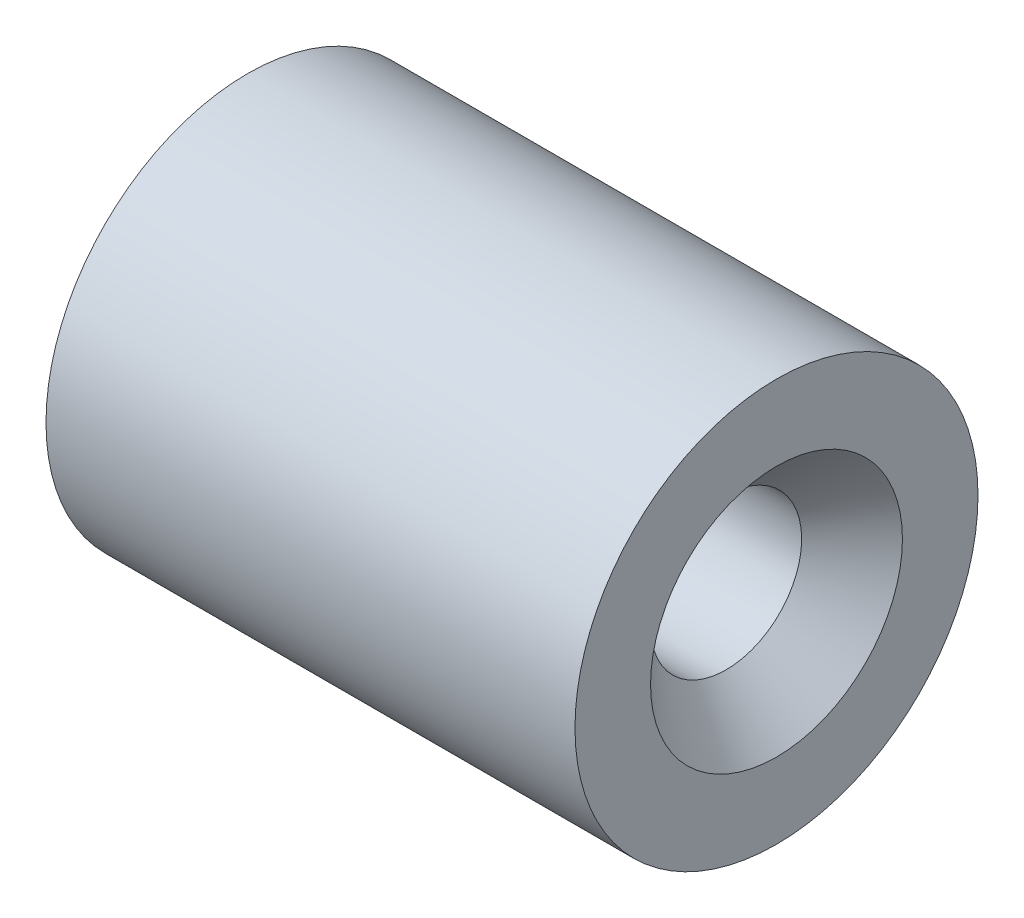
ISO-10303-21;
HEADER;
FILE_DESCRIPTION(('STEP AP214'),'2;1');
FILE_NAME('part.step','',(''),(''),'','','');
FILE_SCHEMA(('AUTOMOTIVE_DESIGN { 1 0 10303 214 1 1 1 1 }'));
ENDSEC;
DATA;
#1=APPLICATION_CONTEXT('core data for automotive mechanical design processes');
#2=APPLICATION_PROTOCOL_DEFINITION('international standard','automotive_design',2000,#1);
#3=PRODUCT_CONTEXT('',#1,'mechanical');
#4=PRODUCT('Part','Part','',(#3));
#5=PRODUCT_RELATED_PRODUCT_CATEGORY('part','',(#4));
#6=PRODUCT_DEFINITION_FORMATION('','',#4);
#7=PRODUCT_DEFINITION_CONTEXT('part definition',#1,'design');
#8=PRODUCT_DEFINITION('design','',#6,#7);
#9=PRODUCT_DEFINITION_SHAPE('','',#8);
#10=(LENGTH_UNIT() NAMED_UNIT(*) SI_UNIT(.MILLI.,.METRE.));
#11=(NAMED_UNIT(*) PLANE_ANGLE_UNIT() SI_UNIT($,.RADIAN.));
#12=(NAMED_UNIT(*) SI_UNIT($,.STERADIAN.) SOLID_ANGLE_UNIT());
#13=UNCERTAINTY_MEASURE_WITH_UNIT(LENGTH_MEASURE(1.E-05),#10,'distance_accuracy_value','');
#14=(GEOMETRIC_REPRESENTATION_CONTEXT(3) GLOBAL_UNCERTAINTY_ASSIGNED_CONTEXT((#13)) GLOBAL_UNIT_ASSIGNED_CONTEXT((#10,
#11,#12)) REPRESENTATION_CONTEXT('',''));
#15=CARTESIAN_POINT('',(0.,0.,0.));
#16=DIRECTION('',(0.,0.,1.));
#17=DIRECTION('',(1.,0.,0.));
#18=AXIS2_PLACEMENT_3D('',#15,#16,#17);
#19=CARTESIAN_POINT('',(0.,16.,0.));
#20=DIRECTION('',(1.,0.,0.));
#21=DIRECTION('',(0.,0.,-1.));
#22=AXIS2_PLACEMENT_3D('',#19,#20,#21);
#23=PLANE('',#22);
#24=CARTESIAN_POINT('',(0.,0.,0.));
#25=DIRECTION('',(1.,0.,0.));
#26=DIRECTION('',(0.,0.,-1.));
#27=AXIS2_PLACEMENT_3D('',#24,#25,#26);
#28=CIRCLE('',#27,16.);
#29=CARTESIAN_POINT('',(0.,0.,-16.));
#30=VERTEX_POINT('',#29);
#31=EDGE_CURVE('E74',#30,#30,#28,.T.);
#32=ORIENTED_EDGE('',*,*,#31,.T.);
#33=EDGE_LOOP('',(#32));
#34=FACE_BOUND('',#33,.T.);
#35=CARTESIAN_POINT('',(0.,0.,0.));
#36=DIRECTION('',(1.,0.,0.));
#37=DIRECTION('',(0.,0.,-1.));
#38=AXIS2_PLACEMENT_3D('',#35,#36,#37);
#39=CIRCLE('',#38,9.99999999999999);
#40=CARTESIAN_POINT('',(0.,0.,-9.99999999999999));
#41=VERTEX_POINT('',#40);
#42=EDGE_CURVE('E49',#41,#41,#39,.T.);
#43=ORIENTED_EDGE('',*,*,#42,.F.);
#44=EDGE_LOOP('',(#43));
#45=FACE_BOUND('',#44,.T.);
#46=ADVANCED_FACE('F39',(#34,#45),#23,.T.);
#47=CARTESIAN_POINT('',(-3.99999999999993,0.,0.));
#48=DIRECTION('',(1.,0.,0.));
#49=DIRECTION('',(0.,0.,-1.));
#50=AXIS2_PLACEMENT_3D('',#47,#48,#49);
#51=CONICAL_SURFACE('',#50,6.,0.785398163397457);
#52=ORIENTED_EDGE('',*,*,#42,.T.);
#53=EDGE_LOOP('',(#52));
#54=FACE_BOUND('',#53,.T.);
#55=CARTESIAN_POINT('',(-3.99999999999993,0.,0.));
#56=DIRECTION('',(1.,0.,0.));
#57=DIRECTION('',(0.,0.,-1.));
#58=AXIS2_PLACEMENT_3D('',#55,#56,#57);
#59=CIRCLE('',#58,6.);
#60=CARTESIAN_POINT('',(-3.99999999999993,0.,-6.));
#61=VERTEX_POINT('',#60);
#62=EDGE_CURVE('E80',#61,#61,#59,.T.);
#63=ORIENTED_EDGE('',*,*,#62,.F.);
#64=EDGE_LOOP('',(#63));
#65=FACE_BOUND('',#64,.T.);
#66=ADVANCED_FACE('F61',(#54,#65),#51,.F.);
#67=CARTESIAN_POINT('',(0.,0.,0.));
#68=DIRECTION('',(1.,0.,0.));
#69=DIRECTION('',(0.,0.,-1.));
#70=AXIS2_PLACEMENT_3D('',#67,#68,#69);
#71=CYLINDRICAL_SURFACE('',#70,6.);
#72=ORIENTED_EDGE('',*,*,#62,.T.);
#73=EDGE_LOOP('',(#72));
#74=FACE_BOUND('',#73,.T.);
#75=CARTESIAN_POINT('',(-38.,0.,0.));
#76=DIRECTION('',(1.,0.,0.));
#77=DIRECTION('',(0.,0.,-1.));
#78=AXIS2_PLACEMENT_3D('',#75,#76,#77);
#79=CIRCLE('',#78,6.);
#80=CARTESIAN_POINT('',(-38.,0.,-6.));
#81=VERTEX_POINT('',#80);
#82=EDGE_CURVE('E76',#81,#81,#79,.T.);
#83=ORIENTED_EDGE('',*,*,#82,.F.);
#84=EDGE_LOOP('',(#83));
#85=FACE_BOUND('',#84,.T.);
#86=ADVANCED_FACE('F69',(#74,#85),#71,.F.);
#87=CARTESIAN_POINT('',(-42.,0.,0.));
#88=DIRECTION('',(-1.,0.,0.));
#89=DIRECTION('',(0.,0.,1.));
#90=AXIS2_PLACEMENT_3D('',#87,#88,#89);
#91=CONICAL_SURFACE('',#90,9.99999999999999,0.78539816339745);
#92=ORIENTED_EDGE('',*,*,#82,.T.);
#93=EDGE_LOOP('',(#92));
#94=FACE_BOUND('',#93,.T.);
#95=CARTESIAN_POINT('',(-42.,0.,0.));
#96=DIRECTION('',(1.,0.,0.));
#97=DIRECTION('',(0.,0.,-1.));
#98=AXIS2_PLACEMENT_3D('',#95,#96,#97);
#99=CIRCLE('',#98,9.99999999999999);
#100=CARTESIAN_POINT('',(-42.,0.,-9.99999999999999));
#101=VERTEX_POINT('',#100);
#102=EDGE_CURVE('E84',#101,#101,#99,.T.);
#103=ORIENTED_EDGE('',*,*,#102,.F.);
#104=EDGE_LOOP('',(#103));
#105=FACE_BOUND('',#104,.T.);
#106=ADVANCED_FACE('F92',(#94,#105),#91,.F.);
#107=CARTESIAN_POINT('',(-42.,9.99999999999999,0.));
#108=DIRECTION('',(-1.,0.,0.));
#109=DIRECTION('',(0.,0.,1.));
#110=AXIS2_PLACEMENT_3D('',#107,#108,#109);
#111=PLANE('',#110);
#112=ORIENTED_EDGE('',*,*,#102,.T.);
#113=EDGE_LOOP('',(#112));
#114=FACE_BOUND('',#113,.T.);
#115=CARTESIAN_POINT('',(-42.,0.,0.));
#116=DIRECTION('',(1.,0.,0.));
#117=DIRECTION('',(0.,0.,-1.));
#118=AXIS2_PLACEMENT_3D('',#115,#116,#117);
#119=CIRCLE('',#118,16.);
#120=CARTESIAN_POINT('',(-42.,0.,-16.));
#121=VERTEX_POINT('',#120);
#122=EDGE_CURVE('E87',#121,#121,#119,.T.);
#123=ORIENTED_EDGE('',*,*,#122,.F.);
#124=EDGE_LOOP('',(#123));
#125=FACE_BOUND('',#124,.T.);
#126=ADVANCED_FACE('F58',(#114,#125),#111,.T.);
#127=CARTESIAN_POINT('',(0.,0.,0.));
#128=DIRECTION('',(1.,0.,0.));
#129=DIRECTION('',(0.,0.,-1.));
#130=AXIS2_PLACEMENT_3D('',#127,#128,#129);
#131=CYLINDRICAL_SURFACE('',#130,16.);
#132=CARTESIAN_POINT('',(-25.2122506354872,-15.8120347946242,-2.44531401239084));
#133=CARTESIAN_POINT('',(-25.0291937886343,-15.7802377691378,-2.65092305369073));
#134=CARTESIAN_POINT('',(-24.8270165707222,-15.7469510879061,-2.83965618359188));
#135=CARTESIAN_POINT('',(-24.3940129775997,-15.6814107746442,-3.18181140856644));
#136=CARTESIAN_POINT('',(-24.1630889448343,-15.6491611596418,-3.33510778841252));
#137=CARTESIAN_POINT('',(-23.6772864838775,-15.5887046837897,-3.60720741451062));
#138=CARTESIAN_POINT('',(-23.4221343309145,-15.56055619488,-3.72553345871184));
#139=CARTESIAN_POINT('',(-22.8972027272664,-15.5115727434981,-3.92448636154121));
#140=CARTESIAN_POINT('',(-22.6274337380606,-15.4907326281005,-4.00513979542278));
#141=CARTESIAN_POINT('',(-22.0375303253731,-15.4558874309351,-4.13776116900106));
#142=CARTESIAN_POINT('',(-21.7159139557151,-15.4433778189234,-4.18360628041937));
#143=CARTESIAN_POINT('',(-21.0691354472211,-15.4322134016024,-4.22459606936221));
#144=CARTESIAN_POINT('',(-20.7439716582686,-15.4335653448538,-4.21971605111272));
#145=CARTESIAN_POINT('',(-20.0867360273089,-15.4502730522473,-4.15814346238691));
#146=CARTESIAN_POINT('',(-19.7548538420133,-15.4661451924096,-4.09954019198436));
#147=CARTESIAN_POINT('',(-19.1058474663541,-15.5105180434682,-3.92830726525795));
#148=CARTESIAN_POINT('',(-18.7887355148005,-15.5390290283631,-3.81563364949357));
#149=CARTESIAN_POINT('',(-18.1830972502326,-15.604450454414,-3.53852762138781));
#150=CARTESIAN_POINT('',(-17.8942927422201,-15.6412641631149,-3.37468352801317));
#151=CARTESIAN_POINT('',(-17.3533292971094,-15.7182742712824,-2.9955087702479));
#152=CARTESIAN_POINT('',(-17.1010910549519,-15.7584630423721,-2.78029229125129));
#153=CARTESIAN_POINT('',(-16.7223148272779,-15.8230523387834,-2.37860669614167));
#154=CARTESIAN_POINT('',(-16.5815916396533,-15.8483324393305,-2.20559852509325));
#155=CARTESIAN_POINT('',(-16.329723644961,-15.8950758880329,-1.838660116444));
#156=CARTESIAN_POINT('',(-16.2185557519715,-15.9165422107921,-1.64474637578843));
#157=CARTESIAN_POINT('',(-16.0315684900969,-15.95338175054,-1.23760478739352));
#158=CARTESIAN_POINT('',(-15.9560816790194,-15.9686974510913,-1.02421652999521));
#159=CARTESIAN_POINT('',(-15.8482874937379,-15.9907456363287,-0.586372832963913));
#160=CARTESIAN_POINT('',(-15.8159307741993,-15.9974879294818,-0.361930346044916));
#161=CARTESIAN_POINT('',(-15.7987195490126,-16.0010666167643,0.0561145240392188));
#162=CARTESIAN_POINT('',(-15.8076594835832,-15.9991972004797,0.249471580355679));
#163=CARTESIAN_POINT('',(-15.858537352962,-15.9886717913303,0.631571761329953));
#164=CARTESIAN_POINT('',(-15.9004748868664,-15.9800158809178,0.820314942015244));
#165=CARTESIAN_POINT('',(-16.0124582656376,-15.9573161344648,1.18139928289));
#166=CARTESIAN_POINT('',(-16.0814525381082,-15.9434746474647,1.35408493559546));
#167=CARTESIAN_POINT('',(-16.2438373439836,-15.9116863781528,1.68708524328798));
#168=CARTESIAN_POINT('',(-16.3372347100243,-15.8937384462504,1.8473964172269));
#169=CARTESIAN_POINT('',(-16.558062508205,-15.852643311298,2.1735055020843));
#170=CARTESIAN_POINT('',(-16.6883346022483,-15.829123756118,2.33732300615423));
#171=CARTESIAN_POINT('',(-16.9701284485413,-15.78059587994,2.64520893882912));
#172=CARTESIAN_POINT('',(-17.121663526567,-15.7555866310328,2.78926486977561));
#173=CARTESIAN_POINT('',(-17.4749321995006,-15.7006819114357,3.08474384502075));
#174=CARTESIAN_POINT('',(-17.6805635501336,-15.6708467060262,3.23151835079295));
#175=CARTESIAN_POINT('',(-18.1106380648434,-15.6141986622566,3.49499161658069));
#176=CARTESIAN_POINT('',(-18.3350941994477,-15.587387938132,3.61166941017937));
#177=CARTESIAN_POINT('',(-18.841650013409,-15.5343805914937,3.83386209168941));
#178=CARTESIAN_POINT('',(-19.1266258963564,-15.5092579884945,3.93309806557114));
#179=CARTESIAN_POINT('',(-19.708977202069,-15.469128307807,4.08809776323773));
#180=CARTESIAN_POINT('',(-20.0063570730227,-15.4541248926541,4.14384574813621));
#181=CARTESIAN_POINT('',(-20.470476858574,-15.4399754911944,4.19611835817934));
#182=CARTESIAN_POINT('',(-20.6355163995783,-15.4367273088066,4.20802200539566));
#183=CARTESIAN_POINT('',(-20.9660971142843,-15.4338345924649,4.21862667037792));
#184=CARTESIAN_POINT('',(-21.1316383228755,-15.4341903151827,4.21732674777969));
#185=CARTESIAN_POINT('',(-21.4620752468231,-15.4385017121068,4.20151444230267));
#186=CARTESIAN_POINT('',(-21.6269707866273,-15.4424583052002,4.18699868694461));
#187=CARTESIAN_POINT('',(-21.9550059470972,-15.4538420855752,4.14478516562503));
#188=CARTESIAN_POINT('',(-22.1181449380966,-15.4612704776173,4.1170828236799));
#189=CARTESIAN_POINT('',(-22.4442488494976,-15.4795102458043,4.04797005992329));
#190=CARTESIAN_POINT('',(-22.6071625041907,-15.4903776163382,4.00633203551978));
#191=CARTESIAN_POINT('',(-22.9287772280785,-15.5150870611522,3.9095482144817));
#192=CARTESIAN_POINT('',(-23.0874763962597,-15.528930453044,3.85439643321268));
#193=CARTESIAN_POINT('',(-23.3992272192826,-15.5591076613257,3.73071307506304));
#194=CARTESIAN_POINT('',(-23.5522825111477,-15.5754398377867,3.6621903004188));
#195=CARTESIAN_POINT('',(-23.8514853179043,-15.6100287743346,3.51182861776661));
#196=CARTESIAN_POINT('',(-23.9976316616052,-15.6282858590454,3.42998746242597));
#197=CARTESIAN_POINT('',(-24.3659257857721,-15.6773098371536,3.20044479918297));
#198=CARTESIAN_POINT('',(-24.5816968077895,-15.7090699442002,3.04248459146562));
#199=CARTESIAN_POINT('',(-24.9844143379776,-15.7726456882748,2.69350539931348));
#200=CARTESIAN_POINT('',(-25.1714022341267,-15.8044611777673,2.50253473700187));
#201=CARTESIAN_POINT('',(-25.4744452092309,-15.8584922607532,2.12986128011572));
#202=CARTESIAN_POINT('',(-25.5972175347388,-15.8813646242114,1.95373694752074));
#203=CARTESIAN_POINT('',(-25.8126460799434,-15.9225527731605,1.58332939290181));
#204=CARTESIAN_POINT('',(-25.9053190125372,-15.9408710859896,1.38905632552127));
#205=CARTESIAN_POINT('',(-26.0552813361623,-15.9709534977595,0.984854519342838));
#206=CARTESIAN_POINT('',(-26.1122854296924,-15.9826646781726,0.774814230854657));
#207=CARTESIAN_POINT('',(-26.1849504384096,-15.9976504893031,0.347434483534122));
#208=CARTESIAN_POINT('',(-26.2006493941815,-16.0009328825712,0.130101927614945));
#209=CARTESIAN_POINT('',(-26.1901332060592,-15.9987505305172,-0.275057255782333));
#210=CARTESIAN_POINT('',(-26.1691030962248,-15.9943677565478,-0.463045653260739));
#211=CARTESIAN_POINT('',(-26.0962829515531,-15.9793861964801,-0.832739112943855));
#212=CARTESIAN_POINT('',(-26.0444797094248,-15.9687847414569,-1.01444144182337));
#213=CARTESIAN_POINT('',(-25.9133257581528,-15.9424791920509,-1.36699386415251));
#214=CARTESIAN_POINT('',(-25.8339842643191,-15.9267768047398,-1.53784756535458));
#215=CARTESIAN_POINT('',(-25.6517547511753,-15.891697579229,-1.86578106635143));
#216=CARTESIAN_POINT('',(-25.5488903447458,-15.8723244291525,-2.0228744618353));
#217=CARTESIAN_POINT('',(-25.3653410309303,-15.8389616864761,-2.2663475056551));
#218=CARTESIAN_POINT('',(-25.2905446802446,-15.8256344920918,-2.3573743162864));
#219=CARTESIAN_POINT('',(-25.2122506354872,-15.8120347946242,-2.44531401239084));
#220=B_SPLINE_CURVE_WITH_KNOTS('',3,(#132,#133,#134,#135,#136,#137,#138,#139,#140,#141,#142,
#143,#144,#145,#146,#147,#148,#149,#150,#151,#152,#153,#154,#155,#156,#157,#158,#159,#160,#161,
#162,#163,#164,#165,#166,#167,#168,#169,#170,#171,#172,#173,#174,#175,#176,#177,#178,#179,#180,
#181,#182,#183,#184,#185,#186,#187,#188,#189,#190,#191,#192,#193,#194,#195,#196,#197,#198,#199,
#200,#201,#202,#203,#204,#205,#206,#207,#208,#209,#210,#211,#212,#213,#214,#215,#216,#217,#218,
#219),.UNSPECIFIED.,.T.,.F.,(4,2,2,2,2,2,2,2,2,2,2,2,2,2,2,2,2,2,2,2,2,2,2,2,2,2,2,2,2,2,2,2,2,
2,2,2,2,2,2,2,2,2,2,4),(0.,0.830998201450665,1.66490069126829,2.50970640092412,3.35391525893971,
4.32484007288671,5.29623760839353,6.30358282327309,7.31174840553202,8.3087249512895,
9.30350582019038,9.97434287642306,10.6446543855953,11.3210958660806,11.9967627606023,
12.5744927168577,13.1522156541014,13.7094131552679,14.2667668339731,14.8963361744486,
15.5263018508906,16.2866810081204,17.0475884500134,17.9523249844315,18.8573888034175,
19.353404800681,19.8494561246734,20.3456340689003,20.8419843214956,21.3468725408816,
21.8519847579263,22.3567655704151,22.8616316476938,23.6661600537746,24.4695205786199,
25.1147061535094,25.7595328697297,26.4094534336011,27.058775233549,27.6236592234394,
28.1887858270091,28.7537235005107,29.3180965458287,29.6735173426813),.UNSPECIFIED.);
#221=CARTESIAN_POINT('',(-25.2122506354872,-15.8120347946242,-2.44531401239084));
#222=VERTEX_POINT('',#221);
#223=EDGE_CURVE('E11',#222,#222,#220,.T.);
#224=ORIENTED_EDGE('',*,*,#223,.F.);
#225=EDGE_LOOP('',(#224));
#226=FACE_BOUND('',#225,.T.);
#227=ORIENTED_EDGE('',*,*,#122,.T.);
#228=EDGE_LOOP('',(#227));
#229=FACE_BOUND('',#228,.T.);
#230=ORIENTED_EDGE('',*,*,#31,.F.);
#231=EDGE_LOOP('',(#230));
#232=FACE_BOUND('',#231,.T.);
#233=ADVANCED_FACE('F54',(#226,#229,#232),#131,.T.);
#234=CARTESIAN_POINT('',(-21.,-13.,0.));
#235=DIRECTION('',(0.,-1.,0.));
#236=DIRECTION('',(1.,0.,0.));
#237=AXIS2_PLACEMENT_3D('',#234,#235,#236);
#238=CONICAL_SURFACE('',#237,0.,1.04719755119659);
#239=ORIENTED_EDGE('',*,*,#223,.T.);
#240=EDGE_LOOP('',(#239));
#241=FACE_BOUND('',#240,.T.);
#242=CARTESIAN_POINT('',(-21.,-13.,0.));
#243=VERTEX_POINT('',#242);
#244=VERTEX_LOOP('',#243);
#245=FACE_BOUND('',#244,.T.);
#246=ADVANCED_FACE('F52',(#241,#245),#238,.F.);
#247=CLOSED_SHELL('',(#46,#66,#86,#106,#126,#233,#246));
#248=MANIFOLD_SOLID_BREP('B2',#247);
#249=ADVANCED_BREP_SHAPE_REPRESENTATION('',(#18,#248),#14);
#250=SHAPE_DEFINITION_REPRESENTATION(#9,#249);
ENDSEC;
END-ISO-10303-21;
